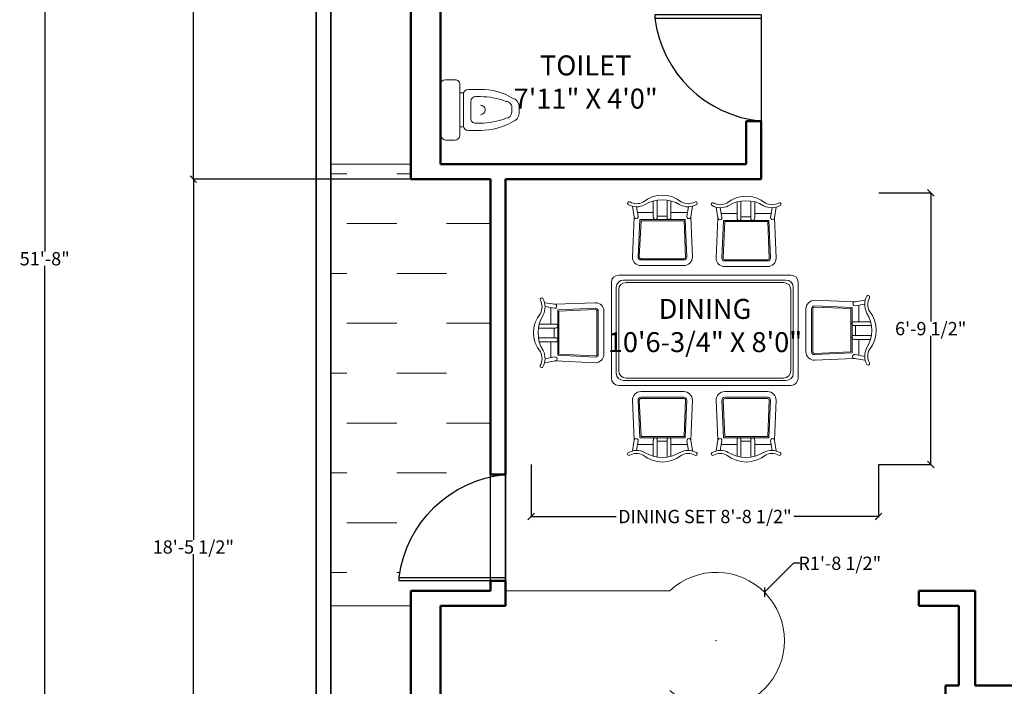
# Model space of a CAD drawing. Units: inches. Extents: x -317284 to 524, y -2236 to 1075.
# Tile 3 of 6: x -24 to 273, y 596 to 796. Entities that reach past the tile are written whole.
import ezdxf

# ---------------------------------------------------------------- set-up
doc = ezdxf.new("R2010")
doc.units = ezdxf.units.IN
doc.header["$MEASUREMENT"] = 0
for name, color, linetype, lineweight in [('A-ANNO-DIMS', 2, 'Continuous', 18), ('A-AREA-IDEN', 7, 'Continuous', 18), ('A-DOOR', 4, 'Continuous', 25), ('A-FLOR-CASE', 8, 'Continuous', 20), ('A-FLOR-FIXT', 9, 'Continuous', 18), ('A-FLOR-PATT', 252, 'Continuous', 13), ('A-FURN', 8, 'Continuous', 18), ('A-WALL', 7, 'Continuous', 50), ('C-PROP', 3, 'Continuous', 35), ('C-SITE-PVMT', 8, 'Continuous', 18)]:
    doc.layers.add(name, color=color, linetype=linetype, lineweight=lineweight)
doc.styles.get("Standard").update_dxf_attribs({"font": 'arial.ttf'})
doc.dimstyles.get("Standard").update_dxf_attribs({"dimtxt": 4, "dimasz": 2, "dimexe": 0.18, "dimexo": 0.0625, "dimgap": 0.09, "dimtad": 0, "dimtih": 1, "dimtoh": 1, "dimdec": 0, "dimzin": 0, "dimdsep": 46, "dimlunit": 4, "dimtxsty": 'Standard', "dimblk": 'OBLIQUE', "dimcen": 0.09, "dimadec": 0, "dimazin": 0, "dimtfac": 1, "dimtdec": 0, "dimtofl": 0, "dimtmove": 0, "dimatfit": 3, "dimldrblk": 'OBLIQUE', "dimfxl": 1, "dimtolj": 1, "dimtzin": 0, "dimarcsym": 0})

# ---------------------------------------------------------------- blocks, each defined once
blk = doc.blocks.new('SDFGHJK')
for p, q in [((282.73, 832.88), (281.73, 832.88)), ((281.73, 832.88), (281.73, 800.88)), ((282.73, 800.88), (282.73, 832.88)), ((282.73, 800.88), (250.73, 800.88))]:
    blk.add_line(p, q)
blk.add_arc((286.22, 797.51), 35.65, 97.2399, 174.5788)
blk = doc.blocks.new('A$C75290641')
for p, q in [((0.7046, 1.4396), (0.7046, 1.5347)), ((0.7276, 1.4396), (0.7276, 1.5396)), ((0.7854, 1.5398), (0.7854, 1.4396)), ((0.8084, 1.5349), (0.8084, 1.4398)), ((1.1969, 1.4338), (1.1969, 1.5289)), ((1.22, 1.4338), (1.22, 1.5339)), ((1.2777, 1.534), (1.2777, 1.4338)), ((1.3008, 1.5291), (1.3008, 1.434)), ((0.5922, 1.4383), (0.5816, 1.5032)), ((0.6153, 1.4439), (0.6047, 1.5002)), ((0.6111, 1.4661), (0.7046, 1.4661)), ((0.8084, 1.4661), (0.9058, 1.4661)), ((0.9114, 1.5002), (0.9021, 1.4439)), ((0.9344, 1.5032), (0.9252, 1.4402)), ((1.0846, 1.4325), (1.074, 1.4974)), ((1.1076, 1.4381), (1.097, 1.4944)), ((1.1034, 1.4603), (1.1969, 1.4603)), ((1.3008, 1.4603), (1.3981, 1.4603)), ((1.4037, 1.4944), (1.3944, 1.4381)), ((1.4268, 1.4974), (1.4175, 1.4344)), ((0.5816, 1.205), (0.5922, 1.4383)), ((0.6148, 1.2054), (0.6253, 1.4258)), ((0.6219, 1.205), (0.6322, 1.4186)), ((0.6253, 1.4258), (0.892, 1.4258)), ((0.6322, 1.4186), (0.8851, 1.4186)), ((0.7276, 1.446), (0.7854, 1.446)), ((0.8851, 1.4186), (0.8941, 1.205)), ((0.892, 1.4258), (0.9013, 1.2053)), ((0.9252, 1.4402), (0.9344, 1.205)), ((1.074, 1.1992), (1.0846, 1.4325)), ((1.1071, 1.1996), (1.1177, 1.42)), ((1.1143, 1.1992), (1.1245, 1.4128)), ((1.1177, 1.42), (1.3844, 1.42)), ((1.1245, 1.4128), (1.3775, 1.4128)), ((1.22, 1.4402), (1.2777, 1.4402)), ((1.3775, 1.4128), (1.3864, 1.1992)), ((1.3844, 1.42), (1.3936, 1.1995)), ((1.4175, 1.4344), (1.4268, 1.1992)), ((0.884, 1.195), (0.632, 1.195)), ((0.884, 1.1878), (0.632, 1.1878)), ((1.3764, 1.1892), (1.1244, 1.1892)), ((1.3764, 1.182), (1.1244, 1.182)), ((0.884, 1.1546), (0.632, 1.1546)), ((1.3764, 1.1488), (1.1244, 1.1488)), ((0.4578, 0.7745), (0.4578, 1.0553)), ((0.501, 1.0985), (1.007, 1.0985)), ((0.5298, 1.0697), (1.007, 1.0697)), ((0.5442, 1.0553), (1.007, 1.0553)), ((1.007, 1.0985), (1.513, 1.0985)), ((1.007, 1.0697), (1.4842, 1.0697)), ((1.007, 1.0553), (1.4698, 1.0553)), ((1.5562, 1.0553), (1.5562, 0.7745)), ((0.4866, 0.7745), (0.4866, 1.0265)), ((0.501, 0.7745), (0.501, 1.0121)), ((1.513, 1.0121), (1.513, 0.7745)), ((1.5274, 1.0265), (1.5274, 0.7745)), ((0.0652, 0.9366), (0.1282, 0.9273)), ((0.1282, 0.9273), (0.3634, 0.9366)), ((1.8873, 0.9416), (1.6521, 0.9509)), ((1.9503, 0.9509), (1.8873, 0.9416)), ((1.9473, 0.9279), (1.891, 0.9186)), ((0.0682, 0.9136), (0.1245, 0.9043)), ((0.1023, 0.8106), (0.1023, 0.908)), ((0.1426, 0.8942), (0.3631, 0.9035)), ((0.1426, 0.6275), (0.1426, 0.8942)), ((0.1498, 0.8873), (0.3634, 0.8963)), ((0.1498, 0.6344), (0.1498, 0.8873)), ((0.3734, 0.8862), (0.3734, 0.6342)), ((0.3806, 0.8862), (0.3806, 0.6342)), ((0.4138, 0.8862), (0.4138, 0.6342)), ((1.6017, 0.9005), (1.6017, 0.6485)), ((1.6349, 0.9005), (1.6349, 0.6485)), ((1.6421, 0.9005), (1.6421, 0.6485)), ((1.8657, 0.9016), (1.6521, 0.9106)), ((1.8729, 0.9085), (1.6524, 0.9178)), ((1.8657, 0.6487), (1.8657, 0.9016)), ((1.8729, 0.6418), (1.8729, 0.9085)), ((1.9132, 0.8249), (1.9132, 0.9222)), ((0.0335, 0.8106), (0.1286, 0.8106)), ((1.9819, 0.8249), (1.8869, 0.8249)), ((0.0286, 0.7876), (0.1288, 0.7876)), ((0.1224, 0.7298), (0.1224, 0.7876)), ((0.4578, 0.7745), (0.4578, 0.4937)), ((0.4866, 0.7745), (0.4866, 0.5225)), ((0.501, 0.7745), (0.501, 0.5369)), ((1.513, 0.5369), (1.513, 0.7745)), ((1.5274, 0.5225), (1.5274, 0.7745)), ((1.5562, 0.4937), (1.5562, 0.7745)), ((1.9869, 0.8019), (1.8867, 0.8019)), ((1.893, 0.7441), (1.893, 0.8019)), ((0.1288, 0.7298), (0.0287, 0.7298)), ((0.1288, 0.7068), (0.0337, 0.7068)), ((0.1023, 0.6133), (0.1023, 0.7068)), ((1.8867, 0.7441), (1.9867, 0.7441)), ((1.8867, 0.7211), (1.9817, 0.7211)), ((1.9132, 0.6276), (1.9132, 0.7211)), ((1.6521, 0.6384), (1.8657, 0.6487)), ((1.6525, 0.6312), (1.8729, 0.6418)), ((0.1301, 0.5944), (0.0652, 0.5838)), ((0.1245, 0.6175), (0.0682, 0.6069)), ((0.3634, 0.5838), (0.1301, 0.5944)), ((0.363, 0.6169), (0.1426, 0.6275)), ((0.3634, 0.6241), (0.1498, 0.6344)), ((1.6521, 0.5981), (1.8854, 0.6087)), ((1.8854, 0.6087), (1.9503, 0.5981)), ((1.891, 0.6317), (1.9473, 0.6211)), ((0.5298, 0.4793), (1.007, 0.4793)), ((0.5442, 0.4937), (1.007, 0.4937)), ((1.007, 0.4937), (1.4698, 0.4937)), ((1.007, 0.4793), (1.4842, 0.4793)), ((0.501, 0.4505), (1.007, 0.4505)), ((0.884, 0.4138), (0.632, 0.4138)), ((1.007, 0.4505), (1.513, 0.4505)), ((1.3764, 0.4138), (1.1244, 0.4138)), ((0.5816, 0.3634), (0.5922, 0.1301)), ((0.6148, 0.363), (0.6253, 0.1426)), ((0.6219, 0.3634), (0.6322, 0.1498)), ((0.884, 0.3806), (0.632, 0.3806)), ((0.884, 0.3734), (0.632, 0.3734)), ((0.8851, 0.1498), (0.8941, 0.3634)), ((0.892, 0.1426), (0.9013, 0.3631)), ((0.9252, 0.1282), (0.9344, 0.3634)), ((1.074, 0.3634), (1.0846, 0.1301)), ((1.1071, 0.363), (1.1177, 0.1426)), ((1.1143, 0.3634), (1.1245, 0.1498)), ((1.3764, 0.3806), (1.1244, 0.3806)), ((1.3764, 0.3734), (1.1244, 0.3734)), ((1.3775, 0.1498), (1.3864, 0.3634)), ((1.3844, 0.1426), (1.3936, 0.3631)), ((1.4175, 0.1282), (1.4268, 0.3634)), ((0.5922, 0.1301), (0.5816, 0.0652)), ((0.6153, 0.1245), (0.6047, 0.0682)), ((0.6253, 0.1426), (0.892, 0.1426)), ((0.6322, 0.1498), (0.8851, 0.1498)), ((0.7046, 0.1288), (0.7046, 0.0337)), ((0.7276, 0.1288), (0.7276, 0.0287)), ((0.7276, 0.1224), (0.7854, 0.1224)), ((0.7854, 0.0286), (0.7854, 0.1288)), ((0.8084, 0.0335), (0.8084, 0.1286)), ((0.9114, 0.0682), (0.9021, 0.1245)), ((0.9344, 0.0652), (0.9252, 0.1282)), ((1.0846, 0.1301), (1.074, 0.0652)), ((1.1076, 0.1245), (1.097, 0.0682)), ((1.1177, 0.1426), (1.3844, 0.1426)), ((1.1245, 0.1498), (1.3775, 0.1498)), ((1.1969, 0.1288), (1.1969, 0.0337)), ((1.22, 0.1288), (1.22, 0.0287)), ((1.22, 0.1224), (1.2777, 0.1224)), ((1.2777, 0.0286), (1.2777, 0.1288)), ((1.3008, 0.0335), (1.3008, 0.1286)), ((1.4037, 0.0682), (1.3944, 0.1245)), ((1.4268, 0.0652), (1.4175, 0.1282)), ((0.6111, 0.1023), (0.7046, 0.1023)), ((0.8084, 0.1023), (0.9058, 0.1023)), ((1.1034, 0.1023), (1.1969, 0.1023)), ((1.3008, 0.1023), (1.3981, 0.1023))]:
    blk.add_line(p, q)
for centre, radius, start, end in [((0.758, 1.391), 0.1774, 50.3459, 129.6541), ((0.5623, 1.5204), 0.00903, 56.57264, 237.72149), ((0.6064, 1.6014), 0.1012, 241.11729, 297.51414), ((0.6064, 1.6014), 0.0832, 240.92111, 297.51414), ((0.7569, 1.3492), 0.1926, 57.31862, 122.68138), ((0.9097, 1.6014), 0.1012, 242.48586, 298.88271), ((0.9097, 1.6014), 0.0832, 242.48586, 298.02197), ((0.9537, 1.5204), 0.00903, 302.27851, 123.42736), ((1.0546, 1.5146), 0.00903, 56.57264, 237.72149), ((1.0987, 1.5956), 0.1012, 241.11729, 297.51414), ((1.0987, 1.5956), 0.0832, 240.92111, 297.51414), ((1.2504, 1.3852), 0.1774, 50.3459, 129.6541), ((1.2492, 1.3434), 0.1926, 57.31862, 122.68138), ((1.402, 1.5956), 0.1012, 242.48586, 298.88271), ((1.402, 1.5956), 0.0832, 242.48586, 298.02197), ((1.4461, 1.5146), 0.00903, 302.27851, 123.42736), ((0.6037, 1.4411), 0.0119, 166.27479, 13.72521), ((0.7161, 1.4373), 0.0117, 168.67477, 11.32523), ((0.7969, 1.4373), 0.0118, 168.80136, 12.20854), ((0.9136, 1.4421), 0.0117, 170.86137, 9.13863), ((1.0961, 1.4353), 0.0119, 166.27479, 13.72521), ((1.2085, 1.4315), 0.0117, 168.67477, 11.32523), ((1.2893, 1.4315), 0.0118, 168.80136, 12.20854), ((1.406, 1.4363), 0.0117, 170.86137, 9.13863), ((0.632, 1.205), 0.0504, 180, 270), ((0.632, 1.205), 0.0173, 180, 270), ((0.632, 1.205), 0.0101, 180, 270), ((0.884, 1.205), 0.0504, 270, 0), ((0.884, 1.205), 0.0173, 270, 0), ((0.884, 1.205), 0.0101, 270, 0), ((1.1244, 1.1992), 0.0504, 180, 270), ((1.1244, 1.1992), 0.0173, 180, 270), ((1.1244, 1.1992), 0.0101, 180, 270), ((1.3764, 1.1992), 0.0504, 270, 0), ((1.3764, 1.1992), 0.0173, 270, 0), ((1.3764, 1.1992), 0.0101, 270, 0), ((0.501, 1.0553), 0.0432, 90, 180), ((0.5298, 1.0265), 0.0432, 90, 180), ((0.5442, 1.0121), 0.0432, 90, 180), ((1.4698, 1.0121), 0.0432, 0, 90), ((1.4842, 1.0265), 0.0432, 0, 90), ((1.513, 1.0553), 0.0432, 0, 90), ((0.048, 0.9559), 0.00903, 32.27851, 213.42736), ((-0.033, 0.9119), 0.0832, 332.48586, 28.02197), ((-0.033, 0.9119), 0.1012, 332.48586, 28.88271), ((0.1263, 0.9158), 0.0117, 260.86137, 99.13863), ((0.3634, 0.8862), 0.0504, 0, 90), ((1.6521, 0.9005), 0.0504, 90, 180), ((1.8892, 0.9301), 0.0117, 80.86137, 279.13863), ((2.0485, 0.9261), 0.1012, 151.11729, 207.51414), ((1.9675, 0.9702), 0.00903, 326.57264, 147.72149), ((2.0485, 0.9261), 0.0832, 151.97803, 207.51414), ((0.1774, 0.7602), 0.1774, 140.3459, 219.6541), ((0.3634, 0.8862), 0.0173, 0, 90), ((0.3634, 0.8862), 0.0101, 0, 90), ((1.6521, 0.9005), 0.0173, 90, 180), ((1.6521, 0.9005), 0.0101, 90, 180), ((1.7963, 0.7733), 0.1926, 327.31862, 32.68138), ((1.8381, 0.7745), 0.1774, 320.3459, 39.6541), ((0.2192, 0.7591), 0.1926, 147.31862, 212.68138), ((0.1311, 0.7991), 0.0118, 258.80136, 102.20854), ((1.8844, 0.8134), 0.0118, 77.79146, 281.19864), ((0.1311, 0.7183), 0.0117, 258.67477, 101.32523), ((1.8844, 0.7326), 0.0117, 78.67477, 281.32523), ((-0.033, 0.6086), 0.0832, 330.92111, 27.51414), ((-0.033, 0.6086), 0.1012, 331.11729, 27.51414), ((1.6521, 0.6485), 0.0504, 180, 270), ((1.6521, 0.6485), 0.0173, 180, 270), ((1.6521, 0.6485), 0.0101, 180, 270), ((2.0485, 0.6228), 0.1012, 152.48586, 208.88271), ((2.0485, 0.6228), 0.0832, 152.48586, 209.07889), ((0.1273, 0.6059), 0.0119, 256.27478, 103.72522), ((0.3634, 0.6342), 0.0101, 270, 0), ((0.3634, 0.6342), 0.0504, 270, 0), ((0.3634, 0.6342), 0.0173, 270, 0), ((1.8882, 0.6202), 0.0119, 76.27478, 283.72522), ((1.9675, 0.5788), 0.00903, 212.27851, 33.42736), ((0.048, 0.5645), 0.00903, 146.57264, 327.72149), ((0.5298, 0.5225), 0.0432, 180, 270), ((0.5442, 0.5369), 0.0432, 180, 270), ((1.4698, 0.5369), 0.0432, 270, 0), ((1.4842, 0.5225), 0.0432, 270, 0), ((0.501, 0.4937), 0.0432, 180, 270), ((1.513, 0.4937), 0.0432, 270, 0), ((0.632, 0.3634), 0.0504, 90, 180), ((0.884, 0.3634), 0.0504, 0, 90), ((1.1244, 0.3634), 0.0504, 90, 180), ((1.3764, 0.3634), 0.0504, 0, 90), ((0.632, 0.3634), 0.0173, 90, 180), ((0.632, 0.3634), 0.0101, 90, 180), ((0.884, 0.3634), 0.0173, 0, 90), ((0.884, 0.3634), 0.0101, 0, 90), ((1.1244, 0.3634), 0.0173, 90, 180), ((1.1244, 0.3634), 0.0101, 90, 180), ((1.3764, 0.3634), 0.0173, 0, 90), ((1.3764, 0.3634), 0.0101, 0, 90), ((0.6037, 0.1273), 0.0119, 346.27479, 193.72521), ((0.7161, 0.1311), 0.0117, 348.67477, 191.32523), ((0.7969, 0.1311), 0.0118, 347.79146, 191.19864), ((0.9136, 0.1263), 0.0117, 350.86137, 189.13863), ((1.0961, 0.1273), 0.0119, 346.27479, 193.72521), ((1.2085, 0.1311), 0.0117, 348.67477, 191.32523), ((1.2893, 0.1311), 0.0118, 347.79146, 191.19864), ((1.406, 0.1263), 0.0117, 350.86137, 189.13863), ((0.6064, -0.033), 0.1012, 62.48586, 118.88271), ((0.9097, -0.033), 0.1012, 61.11729, 117.51414), ((1.0987, -0.033), 0.1012, 62.48586, 118.88271), ((1.402, -0.033), 0.1012, 61.11729, 117.51414), ((0.5623, 0.048), 0.00903, 122.27851, 303.42736), ((0.6064, -0.033), 0.0832, 62.48586, 119.07889), ((0.758, 0.1774), 0.1774, 230.3459, 309.6541), ((0.7569, 0.2192), 0.1926, 237.31862, 302.68138), ((0.9097, -0.033), 0.0832, 61.97803, 117.51414), ((0.9537, 0.048), 0.00903, 236.57264, 57.72149), ((1.0546, 0.048), 0.00903, 122.27851, 303.42736), ((1.0987, -0.033), 0.0832, 62.48586, 119.07889), ((1.2504, 0.1774), 0.1774, 230.3459, 309.6541), ((1.2492, 0.2192), 0.1926, 237.31862, 302.68138), ((1.402, -0.033), 0.0832, 61.97803, 117.51414), ((1.4461, 0.048), 0.00903, 236.57264, 57.72149)]:
    blk.add_arc(centre, radius, start, end)
at = {"flags": 9}
for tag in ['YSIZE', 'XSIZE', 'ZSIZE']:
    blk.add_attdef(tag, (0.9494, 0.7808), '', height=0.0005, rotation=270, dxfattribs=at)
blk = doc.blocks.new('A$C744D6A7D')
for p, q in [((0, 0.5725), (0, 0.6547)), ((0.0432, 0.6979), (0.4969, 0.7022)), ((0.5401, 0.659), (0.5401, 0.5725)), ((0.4969, 0.5293), (0.0432, 0.5293)), ((0.1188, 0.5293), (0.1188, 0.4969)), ((0.4213, 0.4969), (0.4213, 0.5293)), ((0.0864, 0.3427), (0.0864, 0.4537)), ((0.1188, 0.4969), (0.4213, 0.4969)), ((0.1296, 0.4969), (0.4105, 0.4969)), ((0.4537, 0.4537), (0.4537, 0.3427)), ((0.1512, 0.3889), (0.1512, 0.3457)), ((0.1944, 0.4321), (0.3457, 0.4321)), ((0.3889, 0.3889), (0.3889, 0.3457)), ((0.2377, 0), (0.3025, 0)), ((0.2701, 0.0648), (0.2485, 0.0648)), ((0.2701, 0.0648), (0.2917, 0.0648))]:
    blk.add_line(p, q)
for centre, radius, start, end in [((0.0432, 0.6547), 0.0432, 90, 180), ((0.4969, 0.659), 0.0432, 0, 90), ((0.0432, 0.5725), 0.0432, 180, 270), ((0.4969, 0.5725), 0.0432, 270, 0), ((0.1296, 0.4537), 0.0432, 90, 180), ((0.4105, 0.4537), 0.0432, 0, 90), ((0.1944, 0.3889), 0.0432, 90, 180), ((0.3457, 0.3889), 0.0432, 0, 90), ((0.6538, 0.3442), 0.5674, 179.85141, 210.37068), ((0.7683, 0.3457), 0.6171, 180, 201.56859), ((0.2701, 0.3457), 0.0432, 180, 0), ((-0.2282, 0.3457), 0.6171, 338.43141, 0), ((-0.1137, 0.3442), 0.5674, 329.62932, 0.14859), ((0.2485, 0.1188), 0.054, 180, 270), ((0.2917, 0.1188), 0.054, 270, 0), ((0.2377, 0.0756), 0.0756, 193.98485, 270), ((0.3025, 0.0756), 0.0756, 270, 346.01515)]:
    blk.add_arc(centre, radius, start, end)
blk = doc.blocks.new('_Oblique')
at = {"color": 0, "linetype": 'ByBlock', "lineweight": -2}
blk.add_line((-0.5, -0.5), (0.5, 0.5), dxfattribs=at)
blk = doc.blocks.new('*D15')
at = {"layer": 'A-ANNO-DIMS', "color": 0, "lineweight": -2, "transparency": 16777216}
for p, q in [((65.66, 1034.38), (-16.14, 1034.38)), ((-15.96, 1034.38), (-15.96, 726.59)), ((-15.96, 414.53), (-15.96, 722.32)), ((65.66, 414.53), (-16.14, 414.53))]:
    blk.add_line(p, q, dxfattribs=at)
at = {"layer": 'Defpoints', "color": 0, "transparency": 16777216}
for p in [(-15.96, 1034.38), (65.73, 1034.38), (65.73, 414.53)]:
    blk.add_point(p, dxfattribs=at)
at = {"layer": 'A-ANNO-DIMS', "color": 0, "lineweight": -2, "transparency": 16777216, "xscale": 2, "yscale": 2, "zscale": 2}
for p, rotation in [((-15.96, 1034.38), 90), ((-15.96, 414.53), 270)]:
    blk.add_blockref('_Oblique', p, dxfattribs=dict(at, rotation=rotation))
at = {"layer": 'A-ANNO-DIMS', "color": 0, "transparency": 16777216, "insert": (-15.96, 724.45), "char_height": 4, "attachment_point": 5}
blk.add_mtext('\\A1;51\'-8"', dxfattribs=at)
blk = doc.blocks.new('*D29')
at = {"layer": 'A-ANNO-DIMS', "color": 0, "lineweight": -2, "transparency": 16777216}
for p, q in [((130.5, 662.5), (130.5, 646.69)), ((235.11, 662.5), (235.11, 646.69)), ((130.5, 646.87), (156.07, 646.87)), ((235.11, 646.87), (209.54, 646.87))]:
    blk.add_line(p, q, dxfattribs=at)
at = {"layer": 'Defpoints', "color": 0, "transparency": 16777216}
for p in [(130.5, 662.56), (235.11, 662.56), (235.11, 646.87)]:
    blk.add_point(p, dxfattribs=at)
at = {"layer": 'A-ANNO-DIMS', "color": 0, "lineweight": -2, "transparency": 16777216, "xscale": 2, "yscale": 2, "zscale": 2, "rotation": 180}
blk.add_blockref('_Oblique', (130.5, 646.87), dxfattribs=at)
at = {"layer": 'A-ANNO-DIMS', "color": 0, "lineweight": -2, "transparency": 16777216, "xscale": 2, "yscale": 2, "zscale": 2}
blk.add_blockref('_Oblique', (235.11, 646.87), dxfattribs=at)
at = {"layer": 'A-ANNO-DIMS', "color": 0, "transparency": 16777216, "insert": (182.81, 646.87), "char_height": 4, "attachment_point": 5}
blk.add_mtext('\\A1;DINING SET 8\'-8 1/2"', dxfattribs=at)
blk = doc.blocks.new('*D30')
at = {"layer": 'A-ANNO-DIMS', "color": 0, "lineweight": -2, "transparency": 16777216}
for p, q in [((235.17, 744.27), (250.98, 744.27)), ((250.8, 744.27), (250.8, 705.57)), ((250.8, 662.56), (250.8, 701.26)), ((235.17, 662.56), (250.98, 662.56))]:
    blk.add_line(p, q, dxfattribs=at)
at = {"layer": 'Defpoints', "color": 0, "transparency": 16777216}
for p in [(235.11, 744.27), (250.8, 744.27), (235.11, 662.56)]:
    blk.add_point(p, dxfattribs=at)
at = {"layer": 'A-ANNO-DIMS', "color": 0, "lineweight": -2, "transparency": 16777216, "xscale": 2, "yscale": 2, "zscale": 2}
for p, rotation in [((250.8, 744.27), 90), ((250.8, 662.56), 270)]:
    blk.add_blockref('_Oblique', p, dxfattribs=dict(at, rotation=rotation))
at = {"layer": 'A-ANNO-DIMS', "color": 0, "transparency": 16777216, "insert": (250.8, 703.41), "char_height": 4, "attachment_point": 5}
blk.add_mtext('\\A1;6\'-9 1/2"', dxfattribs=at)
blk = doc.blocks.new('*D33')
at = {"layer": 'A-ANNO-DIMS', "color": 0, "lineweight": -2, "transparency": 16777216}
for p, q in [((94.16, 1005.88), (28.6, 1005.88)), ((28.78, 1005.88), (28.78, 879.29)), ((28.78, 748.38), (28.78, 874.97)), ((94.16, 748.38), (28.6, 748.38))]:
    blk.add_line(p, q, dxfattribs=at)
at = {"layer": 'Defpoints', "color": 0, "transparency": 16777216}
for p in [(94.23, 1005.88), (28.78, 748.38), (94.23, 748.38)]:
    blk.add_point(p, dxfattribs=at)
at = {"layer": 'A-ANNO-DIMS', "color": 0, "lineweight": -2, "transparency": 16777216, "xscale": 2, "yscale": 2, "zscale": 2}
for p, rotation in [((28.78, 1005.88), 90), ((28.78, 748.38), 270)]:
    blk.add_blockref('_Oblique', p, dxfattribs=dict(at, rotation=rotation))
at = {"layer": 'A-ANNO-DIMS', "color": 0, "transparency": 16777216, "insert": (28.78, 877.13), "char_height": 4, "attachment_point": 5}
blk.add_mtext('\\A1;21\'-5 1/2"', dxfattribs=at)
blk = doc.blocks.new('*D34')
at = {"layer": 'A-ANNO-DIMS', "color": 0, "lineweight": -2, "transparency": 16777216}
for p, q in [((118.16, 748.38), (28.6, 748.38)), ((28.78, 748.38), (28.78, 639.86)), ((28.78, 527.03), (28.78, 635.55)), ((94.16, 527.03), (28.6, 527.03))]:
    blk.add_line(p, q, dxfattribs=at)
at = {"layer": 'Defpoints', "color": 0, "transparency": 16777216}
for p in [(118.23, 748.38), (28.78, 527.03), (94.23, 527.03)]:
    blk.add_point(p, dxfattribs=at)
at = {"layer": 'A-ANNO-DIMS', "color": 0, "lineweight": -2, "transparency": 16777216, "xscale": 2, "yscale": 2, "zscale": 2}
for p, rotation in [((28.78, 748.38), 90), ((28.78, 527.03), 270)]:
    blk.add_blockref('_Oblique', p, dxfattribs=dict(at, rotation=rotation))
at = {"layer": 'A-ANNO-DIMS', "color": 0, "transparency": 16777216, "insert": (28.78, 637.7), "char_height": 4, "attachment_point": 5}
blk.add_mtext('\\A1;18\'-5 1/2"', dxfattribs=at)
blk = doc.blocks.new('*D55')
at = {"layer": 'A-ANNO-DIMS', "color": 0, "lineweight": -2, "transparency": 16777216}
for p, q in [((209.44, 632.8), (200.74, 624.07)), ((211.44, 632.8), (209.44, 632.8)), ((186.16, 609.53), (186.34, 609.53)), ((186.25, 609.44), (186.25, 609.62))]:
    blk.add_line(p, q, dxfattribs=at)
at = {"layer": 'Defpoints', "color": 0, "transparency": 16777216}
for p in [(200.74, 624.07), (186.25, 609.53)]:
    blk.add_point(p, dxfattribs=at)
at = {"layer": 'A-ANNO-DIMS', "color": 0, "lineweight": -2, "transparency": 16777216, "xscale": 2, "yscale": 2, "zscale": 2, "rotation": 225.0976870737727}
blk.add_blockref('_Oblique', (200.74, 624.07), dxfattribs=at)
at = {"layer": 'A-ANNO-DIMS', "color": 0, "transparency": 16777216, "insert": (223.42, 632.8), "char_height": 4, "attachment_point": 5}
blk.add_mtext('\\A1;R1\'-8 1/2"', dxfattribs=at)

msp = doc.modelspace()

# ---------------------------------------------------------------- hatches: boundary and pattern name
at = {"layer": 'A-FLOR-PATT'}
h = msp.add_hatch(dxfattribs=at)
h.set_pattern_fill('DASH', color=256, scale=120)
h.paths.add_polyline_path([(118.23, 748.38), (94.23, 748.38), (94.23, 752.88), (70.23, 752.88), (70.23, 620.03), (94.23, 620.03), (94.23, 624.53), (118.23, 624.53), (118.23, 627.53), (90.73, 627.53), (90.73, 628.53, -0.315348), (118.23, 658.81), (118.23, 659.53)])

# ---------------------------------------------------------------- linework, layer by layer
at = {"layer": 'A-DOOR'}
for p, q in [((118.23, 627.53), (118.23, 659.53)), ((122.73, 659.53), (122.73, 627.53))]:
    msp.add_line(p, q, dxfattribs=at)
at = {"layer": 'A-FLOR-CASE'}
for p in [(122.73, 624.53), (172.23, 624.53)]:
    msp.add_line(p, (148.23, 624.53), dxfattribs=at)
msp.add_arc((186.25, 609.53), 20.53, 226.9294, 133.0706, dxfattribs=at)
at = {"layer": 'A-WALL'}
for p, q in [((94.23, 876.88), (94.23, 748.38)), ((103.23, 805.38), (103.23, 752.88)), ((103.23, 800.88), (103.23, 752.88)), ((199.73, 765.88), (195.23, 765.88)), ((195.23, 765.88), (195.23, 752.88)), ((199.73, 765.88), (199.73, 748.38)), ((195.23, 752.88), (103.23, 752.88)), ((118.23, 748.38), (94.23, 748.38)), ((118.23, 748.38), (118.23, 659.53)), ((199.73, 748.38), (122.73, 748.38)), ((122.73, 748.38), (122.73, 659.53)), ((122.73, 659.53), (118.23, 659.53)), ((122.73, 627.53), (118.23, 627.53)), ((118.23, 627.53), (118.23, 624.53)), ((122.73, 627.53), (122.73, 620.03)), ((118.23, 624.53), (94.23, 624.53)), ((94.23, 624.53), (94.23, 620.03)), ((247.23, 620.03), (247.23, 624.53)), ((247.23, 624.53), (264.23, 624.53)), ((264.23, 596.03), (264.23, 624.53)), ((94.23, 620.03), (94.23, 536.03)), ((103.23, 620.03), (103.23, 536.03)), ((103.23, 620.03), (103.23, 620.03)), ((103.23, 620.03), (122.73, 620.03)), ((259.23, 620.03), (247.23, 620.03)), ((259.23, 596.03), (259.23, 620.03)), ((255.23, 536.03), (255.23, 596.03)), ((255.23, 596.03), (259.23, 596.03)), ((259.23, 596.03), (255.23, 596.03)), ((398.73, 596.03), (264.23, 596.03))]:
    msp.add_line(p, q, dxfattribs=at)
at = {"layer": 'C-PROP'}
for points in [[(475.23, 1034.38), (475.23, 414.53), (65.73, 414.53), (65.73, 1034.38)], [(470.73, 1029.88), (470.73, 419.03), (70.23, 419.03), (70.23, 1029.88)]]:
    msp.add_lwpolyline(points, close=True, dxfattribs=at)
at = {"layer": 'C-SITE-PVMT'}
for p, q in [((94.23, 752.88), (70.23, 752.88)), ((94.23, 620.03), (70.23, 620.03))]:
    msp.add_line(p, q, dxfattribs=at)

# ---------------------------------------------------------------- block references
at = {"layer": 'A-DOOR', "rotation": 90}
msp.add_blockref('SDFGHJK', (1000.61, 515.15), dxfattribs=at)
at = {"layer": 'A-DOOR', "xscale": -1, "rotation": 90}
msp.add_blockref('SDFGHJK', (923.61, 910.26), dxfattribs=at)
at = {"layer": 'A-FLOR-FIXT', "xscale": 33.64995820618366, "yscale": 33.64995820618366, "zscale": 33.64995820618366, "rotation": 89.99999999999999}
msp.add_blockref('A$C744D6A7D', (126.85, 760.16), dxfattribs=at)
at = {"layer": 'A-FURN', "xscale": 51.20988748181403, "yscale": 51.20988748181403, "zscale": 51.20988748181403}
msp.add_blockref('A$C75290641', (131.2, 663.26), dxfattribs=at)

# ---------------------------------------------------------------- texts
at = {"layer": 'A-AREA-IDEN', "char_height": 6, "attachment_point": 1}
for s, width, insert in [('\\pxqc;TOILET\\P7\'11" X 4\'0"', 67.9596, (112.94, 785.64)), ('\\pxqc;DINING\\P10\'6-3/4" X 8\'0"', 150.999, (107.33, 712.35))]:
    msp.add_mtext_dynamic_manual_height_columns(s, width=width, gutter_width=30, heights=[0], dxfattribs=dict(at, insert=insert))

# ---------------------------------------------------------------- dimensions: what is measured, and where the dimension line sits
at = {"layer": 'A-ANNO-DIMS'}
for base, p1, p2, override, picture, middle in [((-15.96, 1034.38), (65.73, 414.53), (65.73, 1034.38), {"dimclrd": 0, "dimclre": 0, "dimclrt": 0}, '*D15', (-15.96, 724.45)), ((28.78, 748.38), (94.23, 1005.88), (94.23, 748.38), {"dimdec": 1, "dimlfac": 1, "dimrnd": 0, "dimzin": 1, "dimdsep": 46, "dimlunit": 4, "dimfrac": 2}, '*D33', (28.78, 877.13)), ((28.7766, 527.0289), (118.2266, 748.3794), (94.2266, 527.0289), {"dimdec": 1, "dimlfac": 1, "dimrnd": 0, "dimzin": 1, "dimdsep": 46, "dimlunit": 4, "dimfrac": 2}, '*D34', (28.7766, 637.7042)), ((250.8, 744.27), (235.11, 662.56), (235.11, 744.27), {"dimdec": 1, "dimlfac": 1, "dimrnd": 0, "dimzin": 1, "dimdsep": 46, "dimlunit": 4, "dimfrac": 2}, '*D30', (250.8, 703.41))]:
    dim = msp.add_linear_dim(base=base, p1=p1, p2=p2, angle=90, dimstyle='Standard', override=override, dxfattribs=at)
    dim.commit()
    dim.dimension.update_dxf_attribs({"geometry": picture, "text_midpoint": middle})
dim = msp.add_linear_dim(base=(235.11, 646.87), p1=(130.5, 662.56), p2=(235.11, 662.56), text='DINING SET <>', dimstyle='Standard', override={"dimdec": 1, "dimlfac": 1, "dimrnd": 0, "dimzin": 1, "dimdsep": 46, "dimlunit": 4, "dimfrac": 2}, dxfattribs=at)
dim.commit()
dim.dimension.update_dxf_attribs({"geometry": '*D29', "text_midpoint": (182.81, 646.87)})
dim = msp.add_radius_dim(center=(186.25, 609.53), mpoint=(200.74, 624.07), dimstyle='Standard', override={"dimdec": 1, "dimlfac": 1, "dimrnd": 0, "dimzin": 1, "dimdsep": 46, "dimlunit": 4, "dimfrac": 2}, dxfattribs=at)
dim.commit()
dim.dimension.update_dxf_attribs({"geometry": '*D55', "text_midpoint": (223.42, 632.8), "dimtype": 164})

doc.saveas('drawing.dxf')
